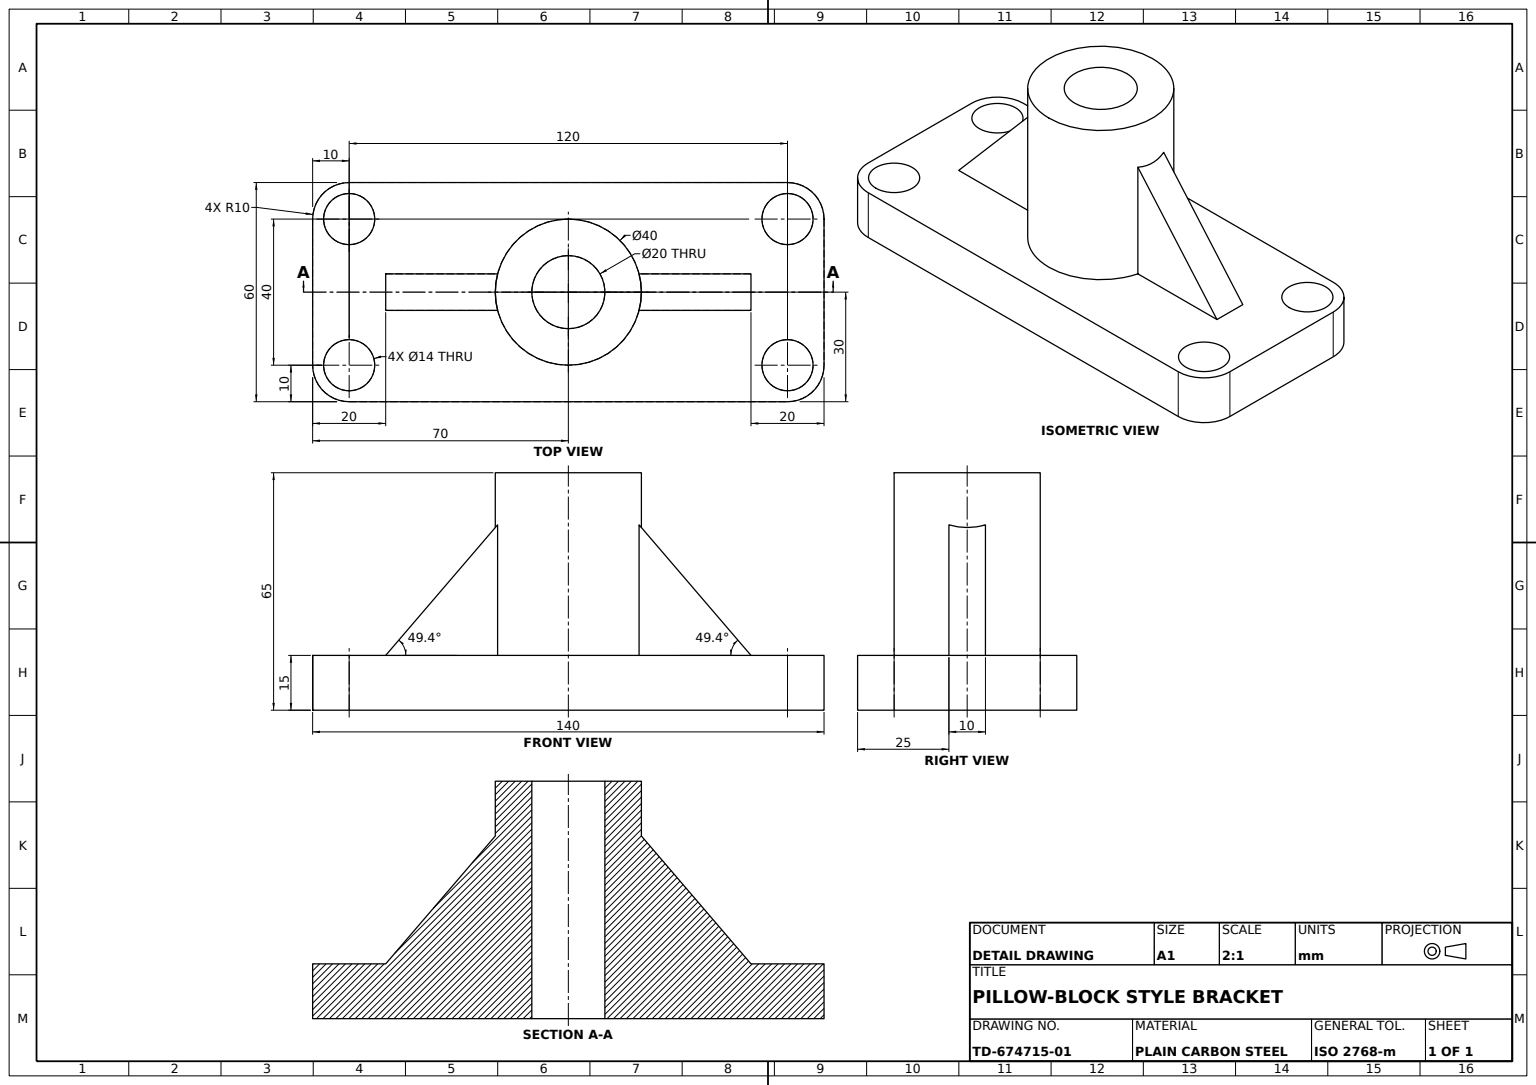
from build123d import *

# Parameters (mm, degrees)
BASE_PLATE_PROFILE_R                 = 7
BASE_PLATE_WITH_MOUNTING_HOLES_DEPTH = 15
BEARING_BOSS_PROFILE_R               = 20
BEARING_BOSS_DEPTH                   = 50
BORE_PROFILE_R                       = 10
BEARING_BORE_DEPTH                   = 243
SUPPORT_RIB_REACH                    = 102.125
SUPPORT_RIB_PROFILE_WALL_W           = 248.347566232
SUPPORT_RIB_PROFILE_WALL_H           = 10


with BuildPart() as part:
    # Base Plate Profile → Base Plate with Mounting Holes (new body)
    with BuildSketch(Plane(origin=(0, 0, 0), x_dir=(1, 0, 0), z_dir=(0, 1, 0))):
        with BuildLine():
            Line((70, 20), (70, -20))
            ThreePointArc((70, -20), (67.071067812, -27.071067812), (60, -30))
            Line((60, -30), (-60, -30))
            ThreePointArc((-60, -30), (-67.071067812, -27.071067812), (-70, -20))
            Line((-70, -20), (-70, 20))
            ThreePointArc((-70, 20), (-67.071067812, 27.071067812), (-60, 30))
            Line((-60, 30), (60, 30))
            ThreePointArc((60, 30), (67.071067812, 27.071067812), (70, 20))
        make_face()
        with Locations(Location((60, -20, 0), (0, 0, 270))):
            Circle(BASE_PLATE_PROFILE_R, mode=Mode.SUBTRACT)
        with Locations(Location((-60, 20, 0), (0, 0, 270))):
            Circle(BASE_PLATE_PROFILE_R, mode=Mode.SUBTRACT)
        with Locations(Location((60, 20, 0), (0, 0, 270))):
            Circle(BASE_PLATE_PROFILE_R, mode=Mode.SUBTRACT)
        with Locations(Location((-60, -20, 0), (0, 0, 270))):
            Circle(BASE_PLATE_PROFILE_R, mode=Mode.SUBTRACT)
    extrude(amount=BASE_PLATE_WITH_MOUNTING_HOLES_DEPTH)

    # Bearing Boss Profile → Bearing Boss (add)
    with BuildSketch(Plane(origin=(0, 15, 0), x_dir=(1, 0, 0), z_dir=(0, 1, 0))):
        with Locations(Location((0, 0, 0), (0, 0, 270))):
            Circle(BEARING_BOSS_PROFILE_R)
    extrude(amount=BEARING_BOSS_DEPTH)

    # Bore Profile → Bearing Bore (cut)
    with BuildSketch(Plane(origin=(0, 65, 0), x_dir=(1, 0, 0), z_dir=(0, 1, 0))):
        with Locations(Location((0, 0, 0), (0, 0, 270))):
            Circle(BORE_PROFILE_R)
    extrude(amount=-BEARING_BORE_DEPTH, mode=Mode.SUBTRACT)

    # Support Rib Profile wall → Support Rib (add, up to next)
    with BuildSketch(Plane(origin=(35, 32.5, 0), x_dir=(0.650791373456, -0.759256602365, 0), z_dir=(0.759256602365, 0.650791373456, 0)), mode=Mode.PRIVATE) as support_rib_sk1:
        Rectangle(SUPPORT_RIB_PROFILE_WALL_W, SUPPORT_RIB_PROFILE_WALL_H)
    support_rib_tool1 = extrude(support_rib_sk1.sketch, amount=-SUPPORT_RIB_REACH, mode=Mode.PRIVATE) - part.part
    support_rib = support_rib_tool1.solids().sort_by_distance((35, 32.5, 0))[0]
    add(support_rib)

    # Support Rib Mirror: Support Rib across plane
    add(support_rib.mirror(Plane(origin=(0, 0, 0), x_dir=(0, 0, 1), z_dir=(1, 0, 0))))


solid = part.part
